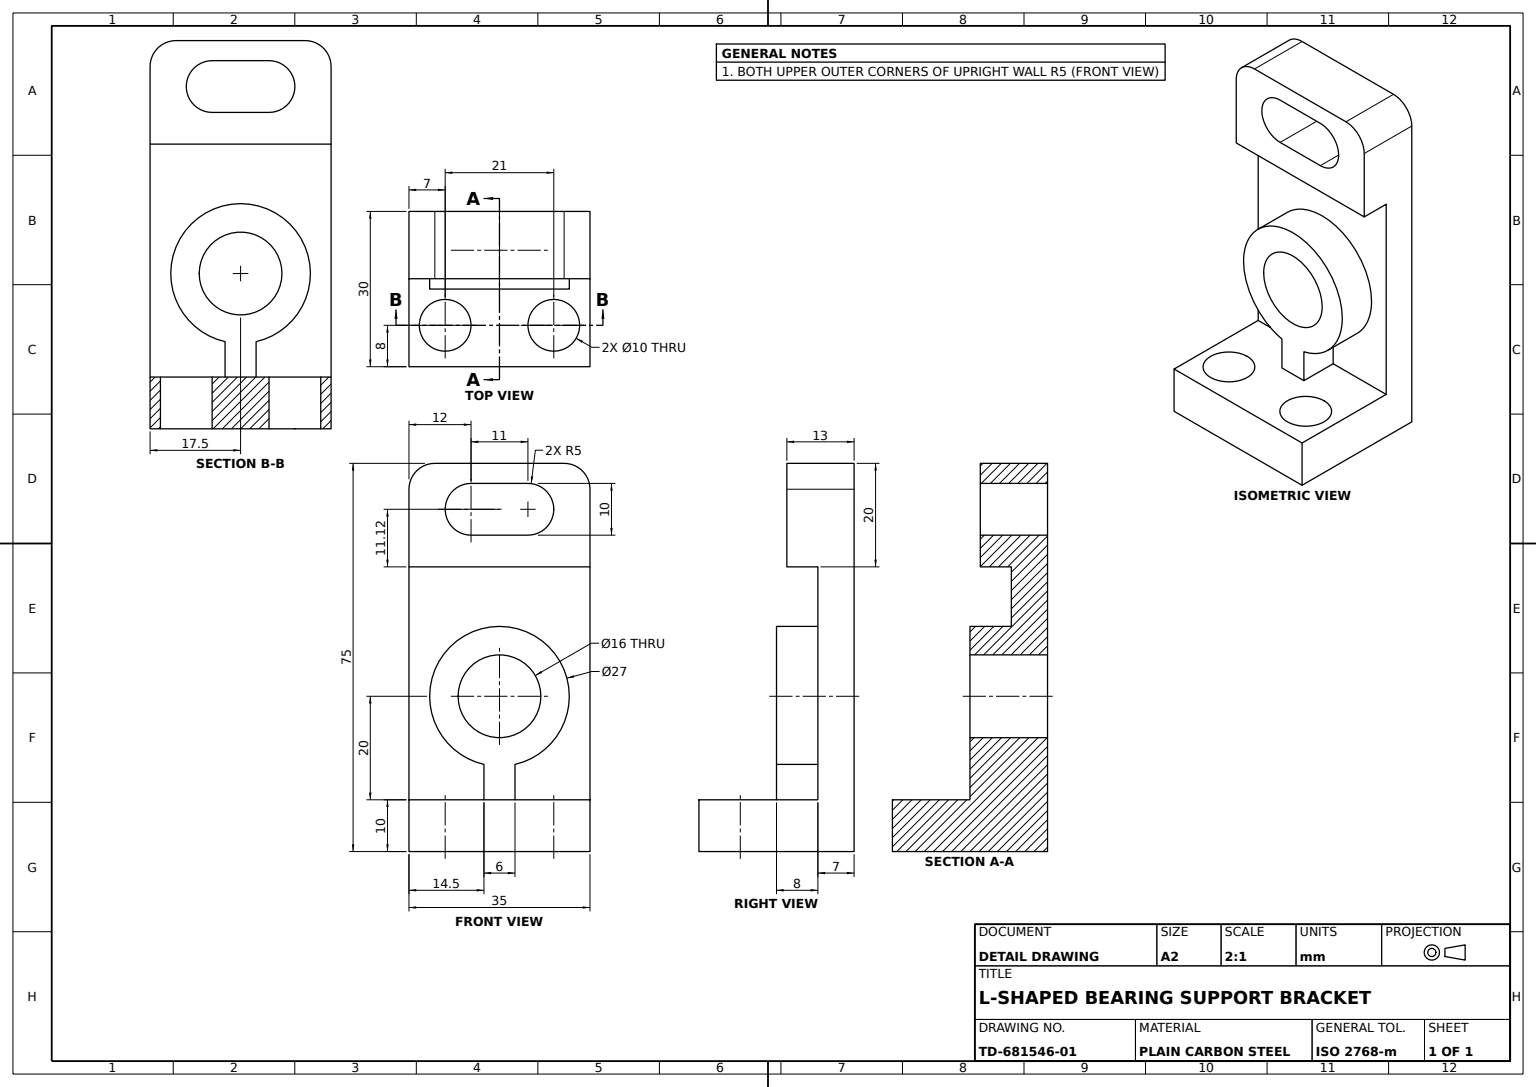
SolidWorks part; units mm, degrees
material "Plain Carbon Steel"
ref_plane "Front Plane" through (0, 0, 0) normal (0, 0, 1) x (1, 0, 0)
ref_plane "Top Plane" through (0, 0, 0) normal (0, 1, 0) x (1, 0, 0)
ref_plane "Right Plane" through (0, 0, 0) normal (1, 0, 0) x (0, 0, -1)
sketch "Base Plate Sketch" plane through (0, 0, 0) normal (0, 1, 0) x (1, 0, 0)
  line L1 (-17.5, 15) -> (17.5, 15)
  line L2 (-17.5, 15) -> (-17.5, -15)
  line L3 (-17.5, -15) -> (17.5, -15)
  line L4 (17.5, 15) -> (17.5, -15)
  line L5 (-17.5, 15) -> (17.5, -15) construction
  line L6 (-17.5, -15) -> (17.5, 15) construction
  point P0 (0, 0)
  dimension "D1" = 30
  dimension "D2" = 35
extrude "Base Plate" add sketch "Base Plate Sketch" along normal blind 10
sketch "Upright Wall Sketch" plane through (0, 10, 0) normal (0, 1, 0) x (1, 0, 0)
  line L0 (-17.5, 15) -> (-17.5, 8)
  line L1 (-17.5, 15) -> (-17.5, -15) construction
  line L2 (-17.5, 8) -> (17.5, 8)
  line L3 (17.5, -15) -> (17.5, 15) construction
  line L4 (17.5, 8) -> (17.5, 15)
  line L5 (17.5, 15) -> (-17.5, 15)
  dimension "D1" = 7
extrude "Upright Wall" add sketch "Upright Wall Sketch" along normal blind 65
sketch "Top Pad Sketch" plane through (0, 0, -8) normal (0, 0, 1) x (1, 0, 0)
  line L0 (-17.5, 55) -> (17.5, 55)
  line L1 (-17.5, 75) -> (-17.5, 10) construction
  line L2 (17.5, 75) -> (17.5, 10) construction
  line L3 (17.5, 55) -> (17.5, 75)
  line L4 (17.5, 75) -> (-17.5, 75)
  line L5 (-17.5, 75) -> (-17.5, 55)
  dimension "D1" = 20
extrude "Top Pad" add sketch "Top Pad Sketch" along normal blind 6
sketch "Wall Mounting Slot Sketch" plane through (0, 0, -2) normal (0, 0, 1) x (1, 0, 0)
  line L0 (-5.5, 66.125) -> (5.5, 66.125) construction
  line L1 (-5.5, 71.125) -> (5.5, 71.125)
  line L2 (-5.5, 61.125) -> (5.5, 61.125)
  line L3 (0, 75) -> (0, 55) construction
  line L4 (17.5, 75) -> (-17.5, 75) construction
  line L5 (-17.5, 55) -> (17.5, 55) construction
  line L7 (-17.5, 55) -> (17.5, 55) construction
  arc A0 (-5.5, 71.125) -> (-5.5, 61.125) centre (-5.5, 66.125) ccw
  arc A1 (5.5, 61.125) -> (5.5, 71.125) centre (5.5, 66.125) ccw
  point P2 (0, 66.125)
  dimension "D1" = 10
  dimension "D2" = 11
  dimension "D3" = 11.125
extrude "Wall Mounting Slot" cut sketch "Wall Mounting Slot Sketch" against normal blind 13
sketch "Bearing Boss Sketch" plane through (0, 0, -8) normal (0, 0, 1) x (1, 0, 0)
  line L0 (-17.5, 10) -> (17.5, 10) construction
  line L1 (-17.5, 55) -> (-17.5, 10) construction
  line L2 (-3, 16.8376) -> (-3, 10)
  line L4 (3, 16.8376) -> (3, 10)
  line L6 (-3, 10) -> (3, 10)
  arc A0 (3, 16.8376) -> (-3, 16.8376) centre (0, 30) ccw
  circle A1 centre (0, 30) radius 8
  dimension "D1" = 27
  dimension "D2" = 16
  dimension "D3" = 20
  dimension "D6" = 6
  dimension "D4" = 14.5
  dimension "D5" = 17.5
extrude "Bearing Boss" add sketch "Bearing Boss Sketch" along normal blind 8
sketch "Base Hole A Sketch" plane through (0, 10, 0) normal (0, 1, 0) x (1, 0, 0)
  line L0 (-17.5, -15) -> (17.5, -15) construction
  line L1 (-17.5, 8) -> (-17.5, -15) construction
  circle A0 centre (-10.5, -7) radius 5
  dimension "D3" = 10
  dimension "D1" = 8
  dimension "D2" = 7
extrude "Base Hole A" cut sketch "Base Hole A Sketch" against normal blind 10
sketch "Base Hole B Sketch" plane through (0, 10, 0) normal (0, 1, 0) x (1, 0, 0)
  line L0 (17.5, -15) -> (17.5, 8) construction
  line L1 (-17.5, -15) -> (17.5, -15) construction
  circle A0 centre (10.5, -7) radius 5
  dimension "D3" = 10
  dimension "D1" = 7
  dimension "D2" = 8
extrude "Base Hole B" cut sketch "Base Hole B Sketch" against normal blind 10
sketch "Bearing Bore Sketch" plane through (0, 0, -8) normal (0, 0, 1) x (1, 0, 0)
  circle A0 centre (0, 30) radius 8
  dimension "D1" = 16
extrude "Bearing Bore" cut sketch "Bearing Bore Sketch" against normal blind 10
fillet "Wall Top Fillet R5 A" radius 5 1 edges at (-17.5, 75, -8.5)
fillet "Wall Top Fillet R5 B" radius 5 1 edges at (17.5, 75, -8.5)
